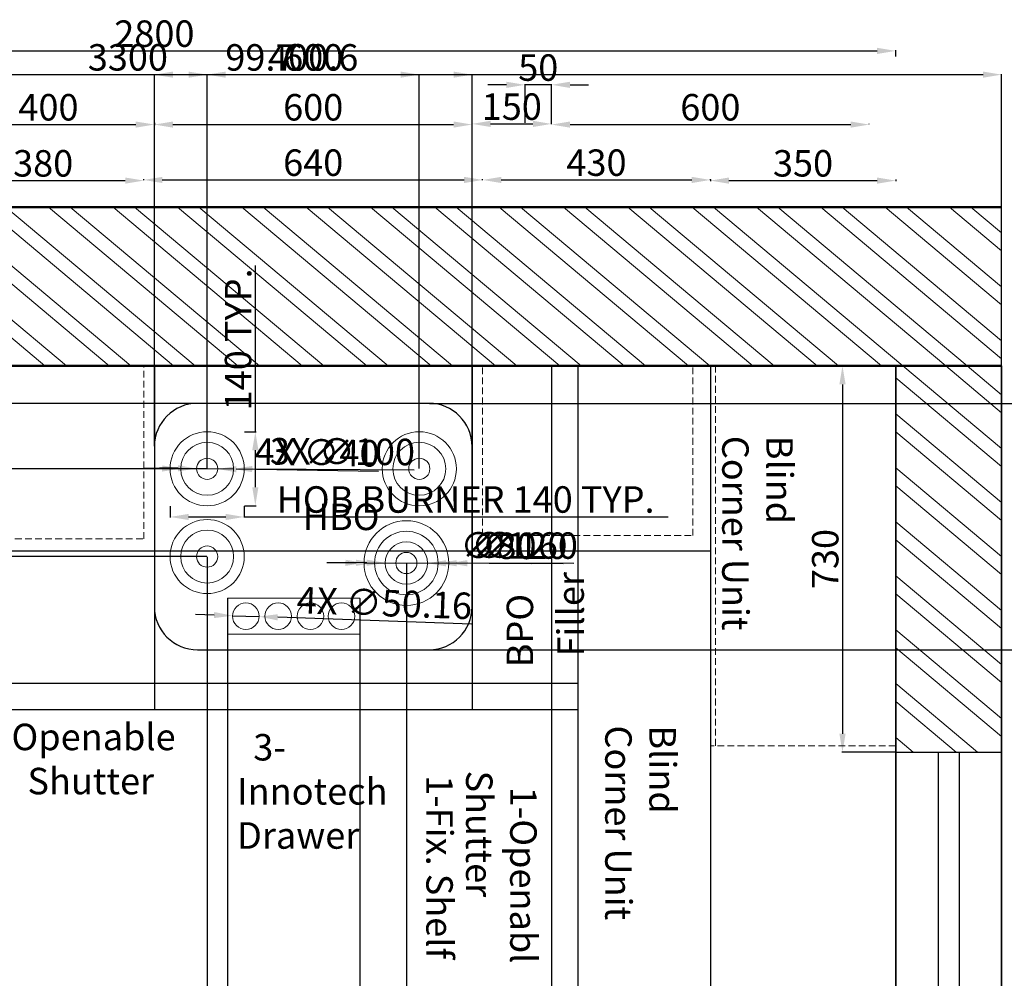
# Model space of a CAD drawing. Units: millimetres. Extents: x 407065 to 421840, y 1168257 to 1177792.
# Tile 9 of 17: x 409170 to 411029, y 1175981 to 1177792. Entities that reach past the tile are written whole.
import ezdxf

# ---------------------------------------------------------------- set-up
doc = ezdxf.new("R2010")
doc.units = ezdxf.units.MM
doc.linetypes.add('DASHED', pattern=[19.05, 12.7, -6.35])
for name, color, linetype, lineweight in [('A-ANNO-DIMS', 6, 'Continuous', 18), ('A-ANNO-TEXT', 30, 'Continuous', 18), ('A-EQPM', 8, 'Continuous', 18), ('A-FURN', 3, 'Continuous', 25), ('A-FURN-HIDN', 7, 'DASHED', 18), ('A-WALL', 7, 'Continuous', 50), ('A-WALL-PATT', 8, 'Continuous', 13)]:
    doc.layers.add(name, color=color, linetype=linetype, lineweight=lineweight)
doc.styles.get("Standard").update_dxf_attribs({"font": 'arial.ttf'})
doc.dimstyles.new('ISO-25', dxfattribs={"dimtxt": 50, "dimasz": 35, "dimexe": 1.25, "dimexo": 0.625, "dimtad": 1, "dimdec": 1, "dimtxsty": 'Standard', "dimcen": 35, "dimadec": 0, "dimazin": 0, "dimtfac": 1, "dimtdec": 1, "dimtmove": 0, "dimatfit": 3, "dimfxl": 1, "dimarcsym": 0})

# ---------------------------------------------------------------- blocks, each defined once
blk = doc.blocks.new('*D4')
at = {"layer": 'A-ANNO-DIMS', "color": 0, "lineweight": -2, "transparency": 16777216}
for p, q in [((409024.3, 1177488.3), (409024.3, 1177488.9)), ((409059.3, 1177487.7), (409369.3, 1177487.7)), ((409404.3, 1177488.3), (409404.3, 1177488.9))]:
    blk.add_line(p, q, dxfattribs=at)
at = {"layer": 'A-ANNO-DIMS', "color": 0, "transparency": 16777216}
for points in [[(409059.3, 1177493.5), (409059.3, 1177481.8), (409024.3, 1177487.7)], [(409369.3, 1177493.5), (409369.3, 1177481.8), (409404.3, 1177487.7)]]:
    blk.add_solid(points, dxfattribs=at)
at = {"layer": 'Defpoints', "color": 0, "transparency": 16777216}
for p in [(409024.3, 1177487.7), (409404.3, 1177487.7), (409404.3, 1177487.7)]:
    blk.add_point(p, dxfattribs=at)
at = {"layer": 'A-ANNO-DIMS', "color": 0, "transparency": 16777216, "insert": (409214.3, 1177513.8), "char_height": 50, "attachment_point": 5}
blk.add_mtext('380', dxfattribs=at)
blk = doc.blocks.new('*D5')
at = {"layer": 'A-ANNO-DIMS', "color": 0, "lineweight": -2, "transparency": 16777216}
for p, q in [((409404.3, 1177488.3), (409404.3, 1177490.2)), ((409439.3, 1177488.9), (410009.3, 1177488.9)), ((410044.3, 1177488.3), (410044.3, 1177490.2))]:
    blk.add_line(p, q, dxfattribs=at)
at = {"layer": 'A-ANNO-DIMS', "color": 0, "transparency": 16777216}
for points in [[(409439.3, 1177494.7), (409439.3, 1177483.1), (409404.3, 1177488.9)], [(410009.3, 1177494.7), (410009.3, 1177483.1), (410044.3, 1177488.9)]]:
    blk.add_solid(points, dxfattribs=at)
at = {"layer": 'Defpoints', "color": 0, "transparency": 16777216}
for p in [(409404.3, 1177487.7), (410044.3, 1177488.9), (410044.3, 1177487.7)]:
    blk.add_point(p, dxfattribs=at)
at = {"layer": 'A-ANNO-DIMS', "color": 0, "transparency": 16777216, "insert": (409724.3, 1177515.1), "char_height": 50, "attachment_point": 5}
blk.add_mtext('640', dxfattribs=at)
blk = doc.blocks.new('*D6')
at = {"layer": 'A-ANNO-DIMS', "color": 0, "lineweight": -2, "transparency": 16777216}
for p, q in [((410044.3, 1177488.3), (410044.3, 1177490.2)), ((410079.3, 1177488.9), (410439.3, 1177488.9)), ((410474.3, 1177488.3), (410474.3, 1177490.2))]:
    blk.add_line(p, q, dxfattribs=at)
at = {"layer": 'A-ANNO-DIMS', "color": 0, "transparency": 16777216}
for points in [[(410079.3, 1177494.7), (410079.3, 1177483.1), (410044.3, 1177488.9)], [(410439.3, 1177494.7), (410439.3, 1177483.1), (410474.3, 1177488.9)]]:
    blk.add_solid(points, dxfattribs=at)
at = {"layer": 'Defpoints', "color": 0, "transparency": 16777216}
for p in [(410044.3, 1177487.7), (410474.3, 1177488.9), (410474.3, 1177487.7)]:
    blk.add_point(p, dxfattribs=at)
at = {"layer": 'A-ANNO-DIMS', "color": 0, "transparency": 16777216, "insert": (410259.3, 1177515.1), "char_height": 50, "attachment_point": 5}
blk.add_mtext('430', dxfattribs=at)
blk = doc.blocks.new('*D7')
at = {"layer": 'A-ANNO-DIMS', "color": 0, "lineweight": -2, "transparency": 16777216}
for p, q in [((410474.3, 1177489.5), (410474.3, 1177486.4)), ((410509.3, 1177487.7), (410789.3, 1177487.7)), ((410824.3, 1177489.5), (410824.3, 1177486.4))]:
    blk.add_line(p, q, dxfattribs=at)
at = {"layer": 'A-ANNO-DIMS', "color": 0, "transparency": 16777216}
for points in [[(410509.3, 1177493.5), (410509.3, 1177481.8), (410474.3, 1177487.7)], [(410789.3, 1177493.5), (410789.3, 1177481.8), (410824.3, 1177487.7)]]:
    blk.add_solid(points, dxfattribs=at)
at = {"layer": 'Defpoints', "color": 0, "transparency": 16777216}
for p in [(410474.3, 1177490.2), (410824.3, 1177490.2), (410824.3, 1177487.7)]:
    blk.add_point(p, dxfattribs=at)
at = {"layer": 'A-ANNO-DIMS', "color": 0, "transparency": 16777216, "insert": (410649.3, 1177513.8), "char_height": 50, "attachment_point": 5}
blk.add_mtext('350', dxfattribs=at)
blk = doc.blocks.new('*D11')
at = {"layer": 'A-ANNO-DIMS', "color": 0, "lineweight": -2, "transparency": 16777216}
for p, q in [((409024.3, 1177596.6), (409024.3, 1177592.3)), ((409059.3, 1177593.5), (409389.3, 1177593.5)), ((409424.3, 1177596.6), (409424.3, 1177592.3))]:
    blk.add_line(p, q, dxfattribs=at)
at = {"layer": 'A-ANNO-DIMS', "color": 0, "transparency": 16777216}
for points in [[(409059.3, 1177599.3), (409059.3, 1177587.7), (409024.3, 1177593.5)], [(409389.3, 1177599.3), (409389.3, 1177587.7), (409424.3, 1177593.5)]]:
    blk.add_solid(points, dxfattribs=at)
at = {"layer": 'Defpoints', "color": 0, "transparency": 16777216}
for p in [(409024.3, 1177597.3), (409424.3, 1177597.3), (409424.3, 1177593.5)]:
    blk.add_point(p, dxfattribs=at)
at = {"layer": 'A-ANNO-DIMS', "color": 0, "transparency": 16777216, "insert": (409224.3, 1177619.7), "char_height": 50, "attachment_point": 5}
blk.add_mtext('400', dxfattribs=at)
blk = doc.blocks.new('*D12')
at = {"layer": 'A-ANNO-DIMS', "color": 0, "lineweight": -2, "transparency": 16777216}
for p, q in [((409424.3, 1177594.1), (409424.3, 1177594.8)), ((409459.3, 1177593.5), (409989.3, 1177593.5)), ((410024.3, 1177594.1), (410024.3, 1177594.8))]:
    blk.add_line(p, q, dxfattribs=at)
at = {"layer": 'A-ANNO-DIMS', "color": 0, "transparency": 16777216}
for points in [[(409459.3, 1177599.3), (409459.3, 1177587.7), (409424.3, 1177593.5)], [(409989.3, 1177599.3), (409989.3, 1177587.7), (410024.3, 1177593.5)]]:
    blk.add_solid(points, dxfattribs=at)
at = {"layer": 'Defpoints', "color": 0, "transparency": 16777216}
for p in [(409424.3, 1177593.5), (410024.3, 1177593.5), (410024.3, 1177593.5)]:
    blk.add_point(p, dxfattribs=at)
at = {"layer": 'A-ANNO-DIMS', "color": 0, "transparency": 16777216, "insert": (409724.3, 1177619.7), "char_height": 50, "attachment_point": 5}
blk.add_mtext('600', dxfattribs=at)
blk = doc.blocks.new('*D13')
at = {"layer": 'A-ANNO-DIMS', "color": 0, "lineweight": -2, "transparency": 16777216}
for p, q in [((410024.3, 1177594.1), (410024.3, 1177596)), ((410059.3, 1177594.8), (410139.3, 1177594.8)), ((410174.3, 1177594.1), (410174.3, 1177596))]:
    blk.add_line(p, q, dxfattribs=at)
at = {"layer": 'A-ANNO-DIMS', "color": 0, "transparency": 16777216}
for points in [[(410059.3, 1177600.6), (410059.3, 1177588.9), (410024.3, 1177594.8)], [(410139.3, 1177600.6), (410139.3, 1177588.9), (410174.3, 1177594.8)]]:
    blk.add_solid(points, dxfattribs=at)
at = {"layer": 'Defpoints', "color": 0, "transparency": 16777216}
for p in [(410024.3, 1177593.5), (410174.3, 1177594.8), (410174.3, 1177593.5)]:
    blk.add_point(p, dxfattribs=at)
at = {"layer": 'A-ANNO-DIMS', "color": 0, "transparency": 16777216, "insert": (410099.3, 1177620.9), "char_height": 50, "attachment_point": 5}
blk.add_mtext('150', dxfattribs=at)
blk = doc.blocks.new('*D14')
at = {"layer": 'A-ANNO-DIMS', "color": 0, "lineweight": -2, "transparency": 16777216}
for p, q in [((410089.3, 1177668.6), (410054.3, 1177668.6)), ((410124.3, 1177596.6), (410124.3, 1177669.8)), ((410174.3, 1177668.6), (410124.3, 1177668.6)), ((410174.3, 1177596.6), (410174.3, 1177669.8)), ((410209.3, 1177668.6), (410244.3, 1177668.6))]:
    blk.add_line(p, q, dxfattribs=at)
at = {"layer": 'A-ANNO-DIMS', "color": 0, "transparency": 16777216}
for points in [[(410089.3, 1177674.4), (410089.3, 1177662.7), (410124.3, 1177668.6)], [(410209.3, 1177674.4), (410209.3, 1177662.7), (410174.3, 1177668.6)]]:
    blk.add_solid(points, dxfattribs=at)
at = {"layer": 'Defpoints', "color": 0, "transparency": 16777216}
for p in [(410124.3, 1177668.6), (410124.3, 1177596), (410174.3, 1177596)]:
    blk.add_point(p, dxfattribs=at)
at = {"layer": 'A-ANNO-DIMS', "color": 0, "transparency": 16777216, "insert": (410149.3, 1177694.7), "char_height": 50, "attachment_point": 5}
blk.add_mtext('50', dxfattribs=at)
blk = doc.blocks.new('*D15')
at = {"layer": 'A-ANNO-DIMS', "color": 0, "lineweight": -2, "transparency": 16777216}
for p, q in [((410174.3, 1177594.1), (410174.3, 1177594.8)), ((410209.3, 1177593.5), (410739.3, 1177593.5)), ((410774.3, 1177594.1), (410774.3, 1177594.8))]:
    blk.add_line(p, q, dxfattribs=at)
at = {"layer": 'A-ANNO-DIMS', "color": 0, "transparency": 16777216}
for points in [[(410209.3, 1177599.3), (410209.3, 1177587.7), (410174.3, 1177593.5)], [(410739.3, 1177599.3), (410739.3, 1177587.7), (410774.3, 1177593.5)]]:
    blk.add_solid(points, dxfattribs=at)
at = {"layer": 'Defpoints', "color": 0, "transparency": 16777216}
for p in [(410174.3, 1177593.5), (410774.3, 1177593.5), (410774.3, 1177593.5)]:
    blk.add_point(p, dxfattribs=at)
at = {"layer": 'A-ANNO-DIMS', "color": 0, "transparency": 16777216, "insert": (410474.3, 1177619.7), "char_height": 50, "attachment_point": 5}
blk.add_mtext('600', dxfattribs=at)
blk = doc.blocks.new('*D16')
at = {"layer": 'A-ANNO-DIMS', "color": 0, "lineweight": -2, "transparency": 16777216}
for p, q in [((408024.3, 1177722.1), (408024.3, 1177733.9)), ((410824.3, 1177722.1), (410824.3, 1177733.9)), ((408059.3, 1177732.7), (410789.3, 1177732.7))]:
    blk.add_line(p, q, dxfattribs=at)
at = {"layer": 'A-ANNO-DIMS', "color": 0, "transparency": 16777216}
for points in [[(408059.3, 1177738.5), (408059.3, 1177726.8), (408024.3, 1177732.7)], [(410789.3, 1177738.5), (410789.3, 1177726.8), (410824.3, 1177732.7)]]:
    blk.add_solid(points, dxfattribs=at)
at = {"layer": 'Defpoints', "color": 0, "transparency": 16777216}
for p in [(408024.3, 1177721.4), (410824.3, 1177732.7), (410824.3, 1177721.4)]:
    blk.add_point(p, dxfattribs=at)
at = {"layer": 'A-ANNO-DIMS', "color": 0, "transparency": 16777216, "insert": (409424.3, 1177758.8), "char_height": 50, "attachment_point": 5}
blk.add_mtext('2800', dxfattribs=at)
blk = doc.blocks.new('*D17')
at = {"layer": 'A-ANNO-DIMS', "color": 0, "lineweight": -2, "transparency": 16777216}
for p, q in [((410828.1, 1177137.8), (410722.6, 1177137.8)), ((410723.8, 1177102.8), (410723.8, 1176442.8)), ((410823.7, 1176407.8), (410722.6, 1176407.8))]:
    blk.add_line(p, q, dxfattribs=at)
at = {"layer": 'A-ANNO-DIMS', "color": 0, "transparency": 16777216}
for points in [[(410718, 1177102.8), (410729.7, 1177102.8), (410723.8, 1177137.8)], [(410718, 1176442.8), (410729.7, 1176442.8), (410723.8, 1176407.8)]]:
    blk.add_solid(points, dxfattribs=at)
at = {"layer": 'Defpoints', "color": 0, "transparency": 16777216}
for p in [(410828.7, 1177137.8), (410723.8, 1176407.8), (410824.3, 1176407.8)]:
    blk.add_point(p, dxfattribs=at)
at = {"layer": 'A-ANNO-DIMS', "color": 0, "transparency": 16777216, "insert": (410697.7, 1176772.8), "char_height": 50, "attachment_point": 5, "rotation": 90}
blk.add_mtext('730', dxfattribs=at)
blk = doc.blocks.new('HOB-BURNER')
for radius in [70, 50, 20]:
    blk.add_circle((409524, 1176943.3), radius)
blk = doc.blocks.new('*D161')
at = {"layer": 'A-ANNO-DIMS', "color": 0, "lineweight": -2, "transparency": 16777216}
for p, q in [((409454, 1176872.7), (409454, 1176851.1)), ((409594, 1176872.7), (409594, 1176851.1)), ((409489, 1176852.3), (409559, 1176852.3)), ((409594, 1176852.3), (410394.9, 1176852.3))]:
    blk.add_line(p, q, dxfattribs=at)
at = {"layer": 'A-ANNO-DIMS', "color": 0, "transparency": 16777216}
for points in [[(409489, 1176858.1), (409489, 1176846.5), (409454, 1176852.3)], [(409559, 1176858.1), (409559, 1176846.5), (409594, 1176852.3)]]:
    blk.add_solid(points, dxfattribs=at)
at = {"layer": 'Defpoints', "color": 0, "transparency": 16777216}
for p in [(409454, 1176873.3), (409594, 1176873.3), (409594, 1176852.3)]:
    blk.add_point(p, dxfattribs=at)
at = {"layer": 'A-ANNO-DIMS', "color": 0, "transparency": 16777216, "insert": (410012, 1176878.8), "char_height": 50, "attachment_point": 5}
blk.add_mtext('HOB BURNER 140 TYP.', dxfattribs=at)
blk = doc.blocks.new('*D162')
at = {"layer": 'A-ANNO-DIMS', "color": 0, "lineweight": -2, "transparency": 16777216}
for p, q in [((409615, 1177013.3), (409615, 1177327.1)), ((409594.6, 1177013.3), (409616.3, 1177013.3)), ((409615, 1176908.3), (409615, 1176978.3)), ((409594.6, 1176873.3), (409616.3, 1176873.3))]:
    blk.add_line(p, q, dxfattribs=at)
at = {"layer": 'A-ANNO-DIMS', "color": 0, "transparency": 16777216}
for points in [[(409609.2, 1176978.3), (409620.8, 1176978.3), (409615, 1177013.3)], [(409609.2, 1176908.3), (409620.8, 1176908.3), (409615, 1176873.3)]]:
    blk.add_solid(points, dxfattribs=at)
at = {"layer": 'Defpoints', "color": 0, "transparency": 16777216}
for p in [(409594, 1177013.3), (409615, 1177013.3), (409594, 1176873.3)]:
    blk.add_point(p, dxfattribs=at)
at = {"layer": 'A-ANNO-DIMS', "color": 0, "transparency": 16777216, "insert": (409588.9, 1177187.7), "char_height": 50, "attachment_point": 5, "rotation": 90}
blk.add_mtext('140 TYP.', dxfattribs=at)
blk = doc.blocks.new('*D165')
at = {"layer": 'A-ANNO-DIMS', "color": 0, "lineweight": -2, "transparency": 16777216}
for p, q in [((407724.3, 1177438.4), (407724.3, 1177689)), ((407759.3, 1177687.8), (410989.3, 1177687.8)), ((411024.3, 1177438.4), (411024.3, 1177689))]:
    blk.add_line(p, q, dxfattribs=at)
at = {"layer": 'A-ANNO-DIMS', "color": 0, "transparency": 16777216}
for points in [[(407759.3, 1177693.6), (407759.3, 1177682), (407724.3, 1177687.8)], [(410989.3, 1177693.6), (410989.3, 1177682), (411024.3, 1177687.8)]]:
    blk.add_solid(points, dxfattribs=at)
at = {"layer": 'Defpoints', "color": 0, "transparency": 16777216}
for p in [(411024.3, 1177687.8), (407724.3, 1177437.8), (411024.3, 1177437.8)]:
    blk.add_point(p, dxfattribs=at)
at = {"layer": 'A-ANNO-DIMS', "color": 0, "transparency": 16777216, "insert": (409374.3, 1177714), "char_height": 50, "attachment_point": 5}
blk.add_mtext('3300', dxfattribs=at)
blk = doc.blocks.new('*D178')
at = {"layer": 'A-ANNO-DIMS', "color": 0, "lineweight": -2, "transparency": 16777216}
for p, q in [((409424.3, 1176986.1), (409424.3, 1177689)), ((409459.3, 1177687.8), (409989.3, 1177687.8)), ((410024.3, 1176986.1), (410024.3, 1177689))]:
    blk.add_line(p, q, dxfattribs=at)
at = {"layer": 'A-ANNO-DIMS', "color": 0, "transparency": 16777216}
for points in [[(409459.3, 1177693.6), (409459.3, 1177682), (409424.3, 1177687.8)], [(409989.3, 1177693.6), (409989.3, 1177682), (410024.3, 1177687.8)]]:
    blk.add_solid(points, dxfattribs=at)
at = {"layer": 'Defpoints', "color": 0, "transparency": 16777216}
for p in [(410024.3, 1177687.8), (409424.3, 1176985.5), (410024.3, 1176985.5)]:
    blk.add_point(p, dxfattribs=at)
at = {"layer": 'A-ANNO-DIMS', "color": 0, "transparency": 16777216, "insert": (409724.3, 1177713.9), "char_height": 50, "attachment_point": 5}
blk.add_mtext('600', dxfattribs=at)
blk = doc.blocks.new('*D179')
at = {"layer": 'A-ANNO-DIMS', "color": 0, "lineweight": -2, "transparency": 16777216}
for p, q in [((409943.6, 1177066.8), (411961.4, 1177066.8)), ((411960.2, 1177031.8), (411960.2, 1176636.4)), ((409943.6, 1176601.4), (411961.4, 1176601.4))]:
    blk.add_line(p, q, dxfattribs=at)
at = {"layer": 'A-ANNO-DIMS', "color": 0, "transparency": 16777216}
for points in [[(411954.3, 1177031.8), (411966, 1177031.8), (411960.2, 1177066.8)], [(411954.3, 1176636.4), (411966, 1176636.4), (411960.2, 1176601.4)]]:
    blk.add_solid(points, dxfattribs=at)
at = {"layer": 'Defpoints', "color": 0, "transparency": 16777216}
for p in [(409943, 1177066.8), (409943, 1176601.4), (411960.2, 1176601.4)]:
    blk.add_point(p, dxfattribs=at)
at = {"layer": 'A-ANNO-DIMS', "color": 0, "transparency": 16777216, "insert": (411934, 1176834.1), "char_height": 50, "attachment_point": 5, "rotation": 90}
blk.add_mtext('465.4', dxfattribs=at)
blk = doc.blocks.new('*D180')
at = {"layer": 'A-ANNO-DIMS', "color": 0, "lineweight": -2, "transparency": 16777216}
for p, q in [((409424.3, 1176986.1), (409424.3, 1177689)), ((409459.3, 1177687.8), (409489, 1177687.8)), ((409524, 1176943.9), (409524, 1177689)), ((409524, 1177687.8), (409690.1, 1177687.8))]:
    blk.add_line(p, q, dxfattribs=at)
at = {"layer": 'A-ANNO-DIMS', "color": 0, "transparency": 16777216}
for points in [[(409459.3, 1177693.6), (409459.3, 1177682), (409424.3, 1177687.8)], [(409489, 1177693.6), (409489, 1177682), (409524, 1177687.8)]]:
    blk.add_solid(points, dxfattribs=at)
at = {"layer": 'Defpoints', "color": 0, "transparency": 16777216}
for p in [(409524, 1177687.8), (409424.3, 1176985.5), (409524, 1176943.3)]:
    blk.add_point(p, dxfattribs=at)
at = {"layer": 'A-ANNO-DIMS', "color": 0, "transparency": 16777216, "insert": (409624.6, 1177713.9), "char_height": 50, "attachment_point": 5}
blk.add_mtext('99.7', dxfattribs=at)
blk = doc.blocks.new('*D181')
at = {"layer": 'A-ANNO-DIMS', "color": 0, "lineweight": -2, "transparency": 16777216}
for p, q in [((409524, 1176943.9), (409524, 1177689)), ((409559, 1177687.8), (409889.6, 1177687.8)), ((409924.6, 1176943.9), (409924.6, 1177689))]:
    blk.add_line(p, q, dxfattribs=at)
at = {"layer": 'A-ANNO-DIMS', "color": 0, "transparency": 16777216}
for points in [[(409559, 1177693.6), (409559, 1177682), (409524, 1177687.8)], [(409889.6, 1177693.6), (409889.6, 1177682), (409924.6, 1177687.8)]]:
    blk.add_solid(points, dxfattribs=at)
at = {"layer": 'Defpoints', "color": 0, "transparency": 16777216}
for p in [(409924.6, 1177687.8), (409524, 1176943.3), (409924.6, 1176943.3)]:
    blk.add_point(p, dxfattribs=at)
at = {"layer": 'A-ANNO-DIMS', "color": 0, "transparency": 16777216, "insert": (409724.3, 1177713.9), "char_height": 50, "attachment_point": 5}
blk.add_mtext('400.6', dxfattribs=at)
blk = doc.blocks.new('*D182')
at = {"layer": 'A-ANNO-DIMS', "color": 0, "lineweight": -2, "transparency": 16777216}
for p, q in [((409505, 1177066.8), (407473.1, 1177066.8)), ((407474.3, 1177031.8), (407474.3, 1176978.3)), ((409523.4, 1176943.3), (407473.1, 1176943.3)), ((407474.3, 1176943.3), (407474.3, 1176742.7))]:
    blk.add_line(p, q, dxfattribs=at)
at = {"layer": 'A-ANNO-DIMS', "color": 0, "transparency": 16777216}
for points in [[(407468.5, 1177031.8), (407480.1, 1177031.8), (407474.3, 1177066.8)], [(407468.5, 1176978.3), (407480.1, 1176978.3), (407474.3, 1176943.3)]]:
    blk.add_solid(points, dxfattribs=at)
at = {"layer": 'Defpoints', "color": 0, "transparency": 16777216}
for p in [(409505.7, 1177066.8), (407474.3, 1176943.3), (409524, 1176943.3)]:
    blk.add_point(p, dxfattribs=at)
at = {"layer": 'A-ANNO-DIMS', "color": 0, "transparency": 16777216, "insert": (407448.1, 1176825.5), "char_height": 50, "attachment_point": 5, "rotation": 90}
blk.add_mtext('123.5', dxfattribs=at)
blk = doc.blocks.new('*D183')
at = {"layer": 'A-ANNO-DIMS', "color": 0, "lineweight": -2, "transparency": 16777216}
for p, q in [((409523.4, 1176943.3), (407473.1, 1176943.3)), ((407474.3, 1176908.3), (407474.3, 1176812.5)), ((409523.4, 1176777.5), (407473.1, 1176777.5)), ((407474.3, 1176777.5), (407474.3, 1176538.4))]:
    blk.add_line(p, q, dxfattribs=at)
at = {"layer": 'A-ANNO-DIMS', "color": 0, "transparency": 16777216}
for points in [[(407468.5, 1176908.3), (407480.1, 1176908.3), (407474.3, 1176943.3)], [(407468.5, 1176812.5), (407480.1, 1176812.5), (407474.3, 1176777.5)]]:
    blk.add_solid(points, dxfattribs=at)
at = {"layer": 'Defpoints', "color": 0, "transparency": 16777216}
for p in [(409524, 1176943.3), (407474.3, 1176777.5), (409524, 1176777.5)]:
    blk.add_point(p, dxfattribs=at)
at = {"layer": 'A-ANNO-DIMS', "color": 0, "transparency": 16777216, "insert": (407448.2, 1176640.4), "char_height": 50, "attachment_point": 5, "rotation": 90}
blk.add_mtext('165.86', dxfattribs=at)
blk = doc.blocks.new('*D184')
at = {"layer": 'A-ANNO-DIMS', "color": 0, "lineweight": -2, "transparency": 16777216}
for p, q in [((409524, 1176776.8), (409524, 1172896.5)), ((409900.3, 1176764.7), (409900.3, 1172896.5)), ((409559, 1172897.8), (409865.3, 1172897.8))]:
    blk.add_line(p, q, dxfattribs=at)
at = {"layer": 'A-ANNO-DIMS', "color": 0, "transparency": 16777216}
for points in [[(409559, 1172903.6), (409559, 1172892), (409524, 1172897.8)], [(409865.3, 1172903.6), (409865.3, 1172892), (409900.3, 1172897.8)]]:
    blk.add_solid(points, dxfattribs=at)
at = {"layer": 'Defpoints', "color": 0, "transparency": 16777216}
for p in [(409524, 1176777.5), (409900.3, 1176765.3), (409900.3, 1172897.8)]:
    blk.add_point(p, dxfattribs=at)
at = {"layer": 'A-ANNO-DIMS', "color": 0, "transparency": 16777216, "insert": (409712.1, 1172924), "char_height": 50, "attachment_point": 5}
blk.add_mtext('376.24', dxfattribs=at)
blk = doc.blocks.new('*D185')
at = {"layer": 'A-ANNO-DIMS', "color": 0, "lineweight": -2, "transparency": 16777216}
for p, q in [((409562.3, 1176698.3), (409562.3, 1172896.5)), ((409812.5, 1176698.3), (409812.5, 1172896.5)), ((409597.3, 1172897.8), (409777.5, 1172897.8))]:
    blk.add_line(p, q, dxfattribs=at)
at = {"layer": 'A-ANNO-DIMS', "color": 0, "transparency": 16777216}
for points in [[(409597.3, 1172903.6), (409597.3, 1172892), (409562.3, 1172897.8)], [(409777.5, 1172903.6), (409777.5, 1172892), (409812.5, 1172897.8)]]:
    blk.add_solid(points, dxfattribs=at)
at = {"layer": 'Defpoints', "color": 0, "transparency": 16777216}
for p in [(409562.3, 1176698.9), (409812.5, 1176698.9), (409812.5, 1172897.8)]:
    blk.add_point(p, dxfattribs=at)
at = {"layer": 'A-ANNO-DIMS', "color": 0, "transparency": 16777216, "insert": (409687.4, 1172923.9), "char_height": 50, "attachment_point": 5}
blk.add_mtext('250.25', dxfattribs=at)
blk = doc.blocks.new('*D224')
at = {"layer": 'A-ANNO-DIMS', "color": 0, "lineweight": -2, "transparency": 16777216}
for p, q in [((409785.3, 1176765.7), (409750.3, 1176765.8)), ((409820.3, 1176765.6), (409980.3, 1176765)), ((410216.2, 1176764.2), (410015.3, 1176764.9))]:
    blk.add_line(p, q, dxfattribs=at)
at = {"layer": 'A-ANNO-DIMS', "color": 0, "transparency": 16777216}
for points in [[(409785.3, 1176771.5), (409785.2, 1176759.8), (409820.3, 1176765.6)], [(410015.3, 1176770.7), (410015.2, 1176759), (409980.3, 1176765)]]:
    blk.add_solid(points, dxfattribs=at)
at = {"layer": 'Defpoints', "color": 0, "transparency": 16777216}
for p in [(409820.3, 1176765.6), (409980.3, 1176765)]:
    blk.add_point(p, dxfattribs=at)
at = {"layer": 'A-ANNO-DIMS', "color": 0, "transparency": 16777216, "insert": (410133.3, 1176792), "char_height": 50, "attachment_point": 5, "rotation": 359.802}
blk.add_mtext('∅160', dxfattribs=at)
blk = doc.blocks.new('*D225')
at = {"layer": 'A-ANNO-DIMS', "color": 0, "lineweight": -2, "transparency": 16777216}
for p, q in [((409805.3, 1176765.7), (409770.3, 1176765.9)), ((409840.3, 1176765.6), (409960.3, 1176765)), ((410196.2, 1176763.9), (409995.3, 1176764.8))]:
    blk.add_line(p, q, dxfattribs=at)
at = {"layer": 'A-ANNO-DIMS', "color": 0, "transparency": 16777216}
for points in [[(409805.3, 1176771.5), (409805.2, 1176759.9), (409840.3, 1176765.6)], [(409995.3, 1176770.7), (409995.2, 1176759), (409960.3, 1176765)]]:
    blk.add_solid(points, dxfattribs=at)
at = {"layer": 'Defpoints', "color": 0, "transparency": 16777216}
for p in [(409840.3, 1176765.6), (409960.3, 1176765)]:
    blk.add_point(p, dxfattribs=at)
at = {"layer": 'A-ANNO-DIMS', "color": 0, "transparency": 16777216, "insert": (410113.4, 1176791.8), "char_height": 50, "attachment_point": 5, "rotation": 359.7357}
blk.add_mtext('∅120', dxfattribs=at)
blk = doc.blocks.new('*D226')
at = {"layer": 'A-ANNO-DIMS', "color": 0, "lineweight": -2, "transparency": 16777216}
for p, q in [((409825.3, 1176765.8), (409790.3, 1176766)), ((409860.3, 1176765.6), (409940.3, 1176765)), ((410137.4, 1176763.6), (409975.3, 1176764.8))]:
    blk.add_line(p, q, dxfattribs=at)
at = {"layer": 'A-ANNO-DIMS', "color": 0, "transparency": 16777216}
for points in [[(409825.3, 1176771.6), (409825.2, 1176760), (409860.3, 1176765.6)], [(409975.3, 1176770.6), (409975.2, 1176758.9), (409940.3, 1176765)]]:
    blk.add_solid(points, dxfattribs=at)
at = {"layer": 'Defpoints', "color": 0, "transparency": 16777216}
for p in [(409860.3, 1176765.6), (409940.3, 1176765)]:
    blk.add_point(p, dxfattribs=at)
at = {"layer": 'A-ANNO-DIMS', "color": 0, "transparency": 16777216, "insert": (410074, 1176791.6), "char_height": 50, "attachment_point": 5, "rotation": 359.6026}
blk.add_mtext('∅80', dxfattribs=at)
blk = doc.blocks.new('*D227')
at = {"layer": 'A-ANNO-DIMS', "color": 0, "lineweight": -2, "transparency": 16777216}
for p, q in [((409439, 1176943.9), (409404, 1176944.1)), ((409474, 1176943.6), (409574, 1176943)), ((409914.7, 1176940.8), (409609, 1176942.8))]:
    blk.add_line(p, q, dxfattribs=at)
at = {"layer": 'A-ANNO-DIMS', "color": 0, "transparency": 16777216}
for points in [[(409439.1, 1176949.7), (409439, 1176938), (409474, 1176943.6)], [(409609.1, 1176948.6), (409609, 1176936.9), (409574, 1176943)]]:
    blk.add_solid(points, dxfattribs=at)
at = {"layer": 'Defpoints', "color": 0, "transparency": 16777216}
for p in [(409474, 1176943.6), (409574, 1176943)]:
    blk.add_point(p, dxfattribs=at)
at = {"layer": 'A-ANNO-DIMS', "color": 0, "transparency": 16777216, "insert": (409779.5, 1176969.3), "char_height": 50, "attachment_point": 5, "rotation": 359.6376}
blk.add_mtext('3X ∅100', dxfattribs=at)
blk = doc.blocks.new('*D228')
at = {"layer": 'A-ANNO-DIMS', "color": 0, "lineweight": -2, "transparency": 16777216}
for p, q in [((409469, 1176944.2), (409434, 1176944.7)), ((409504, 1176943.6), (409544, 1176943)), ((409847.9, 1176938.2), (409579, 1176942.4))]:
    blk.add_line(p, q, dxfattribs=at)
at = {"layer": 'A-ANNO-DIMS', "color": 0, "transparency": 16777216}
for points in [[(409469.1, 1176950), (409468.9, 1176938.4), (409504, 1176943.6)], [(409579.1, 1176948.3), (409578.9, 1176936.6), (409544, 1176943)]]:
    blk.add_solid(points, dxfattribs=at)
at = {"layer": 'Defpoints', "color": 0, "transparency": 16777216}
for p in [(409504, 1176943.6), (409544, 1176943)]:
    blk.add_point(p, dxfattribs=at)
at = {"layer": 'A-ANNO-DIMS', "color": 0, "transparency": 16777216, "insert": (409731.4, 1176967.6), "char_height": 50, "attachment_point": 5, "rotation": 359.0937}
blk.add_mtext('4X ∅40', dxfattribs=at)
blk = doc.blocks.new('*D231')
at = {"layer": 'A-ANNO-DIMS', "color": 0, "lineweight": -2, "transparency": 16777216}
for p, q in [((409537.1, 1176667), (409502.1, 1176668.2)), ((409572.1, 1176665.8), (409622.2, 1176664)), ((410023.1, 1176649.9), (409657.2, 1176662.8))]:
    blk.add_line(p, q, dxfattribs=at)
at = {"layer": 'A-ANNO-DIMS', "color": 0, "transparency": 16777216}
for points in [[(409537.3, 1176672.8), (409536.9, 1176661.2), (409572.1, 1176665.8)], [(409657.4, 1176668.6), (409657, 1176656.9), (409622.2, 1176664)]]:
    blk.add_solid(points, dxfattribs=at)
at = {"layer": 'Defpoints', "color": 0, "transparency": 16777216}
for p in [(409572.1, 1176665.8), (409622.2, 1176664)]:
    blk.add_point(p, dxfattribs=at)
at = {"layer": 'A-ANNO-DIMS', "color": 0, "transparency": 16777216, "insert": (409858.6, 1176683.3), "char_height": 50, "attachment_point": 5, "rotation": 357.9867}
blk.add_mtext('4X ∅50.16', dxfattribs=at)

msp = doc.modelspace()

# ---------------------------------------------------------------- hatches: boundary and pattern name
at = {"layer": 'A-WALL-PATT'}
h = msp.add_hatch(dxfattribs=at)
h.set_pattern_fill('ANSI32', color=256, scale=8.2, angle=95)
h.paths.add_polyline_path([(411024.3133, 1177437.7952), (407724.3133, 1177437.7952), (407724.3133, 1177137.7952), (408024.3133, 1177137.7952), (410824.3133, 1177137.7952), (411024.3133, 1177137.7952)])
h = msp.add_hatch(dxfattribs=at)
h.set_pattern_fill('ANSI32', color=256, scale=8.2, angle=95)
h.paths.add_polyline_path([(411024.3133, 1177137.7952), (410824.3133, 1177137.7952), (410824.3133, 1176407.7952), (411024.3133, 1176407.7952)])

# ---------------------------------------------------------------- linework, layer by layer
at = {"layer": 'A-EQPM'}
msp.add_lwpolyline([(409562.2649, 1176698.8834), (409812.5157, 1176698.8834), (409812.5157, 1176630.8621), (409562.2649, 1176630.8621)], close=True, dxfattribs=at)
for centre, radius in [((409900.2591, 1176765.2756), 80), ((409900.2591, 1176765.2756), 60), ((409900.2591, 1176765.2756), 40), ((409900.2591, 1176765.2756), 20), ((409597.1727, 1176664.8727), 25.0815), ((409658.1191, 1176664.8727), 25.0815), ((409719.0314, 1176664.8727), 25.0815), ((409777.7101, 1176664.8727), 25.0815)]:
    msp.add_circle(centre, radius, dxfattribs=at)
at = {"layer": 'A-FURN'}
for p, q in [((411024.3133, 1174717.7952), (411024.3133, 1177437.7952)), ((409424.3133, 1177137.7952), (409424.3133, 1176487.7952)), ((410024.3133, 1177137.7952), (410024.3133, 1176487.7952)), ((410174.3133, 1177137.7952), (410174.3133, 1174737.7952)), ((410224.3133, 1177137.7952), (410224.3133, 1174737.7952)), ((410474.3133, 1177137.7952), (410474.3133, 1174737.7952)), ((410824.3133, 1177137.7952), (410824.3133, 1174717.7952)), ((410824.3133, 1174717.7952), (410824.3133, 1177137.7952)), ((411024.3133, 1177137.7952), (411024.3133, 1174717.7952)), ((410474.3133, 1176787.7952), (408374.3133, 1176787.7952)), ((410224.3133, 1176537.7952), (408524.3133, 1176537.7952)), ((410224.3133, 1176487.7952), (408524.3133, 1176487.7952)), ((410904.3133, 1176407.7952), (410904.3133, 1175477.7952)), ((410944.3133, 1176407.7952), (410944.3133, 1175477.7952))]:
    msp.add_line(p, q, dxfattribs=at)
for points in [[(409942.9713, 1177066.8168), (409505.6554, 1177066.8168, 0.414213562), (409424.3133, 1176985.4747)], [(410024.3133, 1176682.7483), (410024.3133, 1176985.4747, 0.414213562), (409942.9713, 1177066.8168)], [(409424.3133, 1176985.4747), (409424.3133, 1176682.7483, 0.414213562), (409505.6554, 1176601.4062)], [(409505.6554, 1176601.4062), (409942.9713, 1176601.4062, 0.414213562), (410024.3133, 1176682.7483)]]:
    msp.add_lwpolyline(points, format="xyb", dxfattribs=at)
msp.add_lwpolyline([(410824.3133, 1176407.7952), (411024.3133, 1176407.7952), (411024.3133, 1175477.7952), (410824.3133, 1175477.7952)], close=True, dxfattribs=at)
at = {"layer": 'A-FURN-HIDN'}
for p, q in [((409404.3149, 1176811.0044), (409404.3149, 1177137.7952)), ((410044.3149, 1176817.3455), (410044.3149, 1177137.7952)), ((410441.4631, 1176817.3455), (410441.4631, 1177137.7952)), ((410484.3133, 1177137.7952), (410484.3133, 1176419.9871)), ((408646.6902, 1176811.0192), (409404.3149, 1176811.0044)), ((410044.3149, 1176817.3455), (410441.4631, 1176817.3455)), ((410824.3133, 1176419.9871), (410474.3133, 1176419.9871))]:
    msp.add_line(p, q, dxfattribs=at)
at = {"layer": 'A-WALL'}
for p, q in [((411024.3133, 1177437.7952), (407724.3133, 1177437.7952)), ((410824.3133, 1177137.7952), (408024.3133, 1177137.7952)), ((410824.3133, 1177137.7952), (411024.3133, 1177137.7952))]:
    msp.add_line(p, q, dxfattribs=at)

# ---------------------------------------------------------------- block references
at = {"layer": 'A-EQPM'}
for p in [(0, 0), (400.5954, 0), (0, -165.8625)]:
    msp.add_blockref('HOB-BURNER', p, dxfattribs=at)

# ---------------------------------------------------------------- texts
at = {"layer": 'A-ANNO-TEXT', "char_height": 50, "attachment_point": 1}
for s, width, insert, rotation in [('Blind Corner Unit', 382.409863, (410630.0286, 1177005.5683), 270), ('     Filler', 382.409863, (410185.397, 1176512.3886), 90), ('  BPO', 382.409863, (410089.5949, 1176537.7952), 90), ('Blind Corner Unit', 382.409863, (410409.1375, 1176458.4622), 270), (' 1-Fix. Shelf', 382.409863, (409987.8815, 1176379.7197), 270), ('  1-Openabl Shutter', 534.084465, (410146.2728, 1176373.2573), 270)]:
    msp.add_mtext_dynamic_manual_height_columns(s, width=width, gutter_width=12.5, heights=[0], dxfattribs=dict(at, insert=insert, rotation=rotation))
for s, insert in [('HBO', (409704.4285, 1176877.4788)), ('  1-Openable\\P      Shutter', (409092.9692, 1176461.7378)), ('  3- Innotech Drawer', (409580.4835, 1176442.255))]:
    msp.add_mtext_dynamic_manual_height_columns(s, width=382.409863, gutter_width=12.5, heights=[0], dxfattribs=dict(at, insert=insert))

# ---------------------------------------------------------------- dimensions: what is measured, and where the dimension line sits
at = {"layer": 'A-ANNO-DIMS'}
for base, p1, p2, override, picture, middle in [((410824.3133, 1177732.6671), (408024.3133, 1177721.4288), (410824.3133, 1177721.4288), {"dimclrd": 0, "dimclre": 0, "dimclrt": 0}, '*D16', (409424.3133, 1177758.8207)), ((411024.3133, 1177687.7952), (407724.3133, 1177437.7952), (411024.3133, 1177437.7952), {"dimdec": 0, "dimlfac": 1, "dimrnd": 0, "dimzin": 0, "dimdsep": 46, "dimlunit": 2}, '*D165', (409374.3133, 1177713.9659)), ((410024.3133, 1177687.7952), (409424.3133, 1176985.4747), (410024.3133, 1176985.4747), {"dimdec": 0, "dimlfac": 1, "dimrnd": 0, "dimzin": 0, "dimdsep": 46, "dimlunit": 2}, '*D178', (409724.3133, 1177713.9489)), ((409524.0157, 1177687.7952), (409424.3133, 1176985.4747), (409524.0157, 1176943.3161), {"dimdec": 1, "dimlfac": 1, "dimrnd": 0, "dimzin": 0, "dimdsep": 46, "dimlunit": 2}, '*D180', (409624.5793, 1177713.9489)), ((409924.611, 1177687.7952), (409524.0157, 1176943.3161), (409924.611, 1176943.3161), {"dimdec": 1, "dimlfac": 1, "dimrnd": 0, "dimzin": 0, "dimdsep": 46, "dimlunit": 2}, '*D181', (409724.3133, 1177713.9489)), ((409424.3133, 1177593.5123), (409024.3133, 1177597.2623), (409424.3133, 1177597.2623), {"dimclrd": 0, "dimclre": 0, "dimclrt": 0}, '*D11', (409224.3133, 1177619.666)), ((410024.3133, 1177593.5123), (409424.3133, 1177593.5123), (410024.3133, 1177593.5123), {"dimclrd": 0, "dimclre": 0, "dimclrt": 0}, '*D12', (409724.3133, 1177619.666)), ((410174.3133, 1177594.7623), (410024.3133, 1177593.5123), (410174.3133, 1177593.5123), {"dimclrd": 0, "dimclre": 0, "dimclrt": 0}, '*D13', (410099.3133, 1177620.916)), ((410774.3133, 1177593.5123), (410174.3133, 1177593.5123), (410774.3133, 1177593.5123), {"dimclrd": 0, "dimclre": 0, "dimclrt": 0}, '*D15', (410474.3133, 1177619.666)), ((410044.3149, 1177488.9032), (409404.3149, 1177487.6532), (410044.3149, 1177487.6532), {"dimclrd": 0, "dimclre": 0, "dimclrt": 0}, '*D5', (409724.3149, 1177515.0568)), ((410474.3133, 1177488.9032), (410044.3149, 1177487.6532), (410474.3133, 1177487.6532), {"dimclrd": 0, "dimclre": 0, "dimclrt": 0}, '*D6', (410259.3141, 1177515.0739)), ((409404.3149, 1177487.6532), (409024.3133, 1177487.6532), (409404.3149, 1177487.6532), {"dimclrd": 0, "dimclre": 0, "dimclrt": 0}, '*D4', (409214.3141, 1177513.8239)), ((410824.3133, 1177487.6532), (410474.3133, 1177490.1532), (410824.3133, 1177490.1532), {"dimclrd": 0, "dimclre": 0, "dimclrt": 0}, '*D7', (410649.3133, 1177513.8239)), ((409900.2591, 1172897.7952), (409524.0157, 1176777.4536), (409900.2591, 1176765.2756), {"dimdec": 2, "dimlfac": 1, "dimrnd": 0, "dimzin": 0, "dimdsep": 46, "dimlunit": 2}, '*D184', (409712.1374, 1172923.9659)), ((409812.5157, 1172897.7952), (409562.2649, 1176698.8834), (409812.5157, 1176698.8834), {"dimdec": 2, "dimlfac": 1, "dimrnd": 0, "dimzin": 0, "dimdsep": 46, "dimlunit": 2}, '*D185', (409687.3903, 1172923.9489))]:
    dim = msp.add_linear_dim(base=base, p1=p1, p2=p2, dimstyle='ISO-25', override=override, dxfattribs=at)
    dim.commit()
    dim.dimension.update_dxf_attribs({"geometry": picture, "text_midpoint": middle})
dim = msp.add_linear_dim(base=(410124.3133, 1177668.5564), p1=(410174.3133, 1177596.0123), p2=(410124.3133, 1177596.0123), dimstyle='ISO-25', override={"dimclrd": 0, "dimclre": 0, "dimclrt": 0}, dxfattribs=at)
dim.commit()
dim.dimension.update_dxf_attribs({"geometry": '*D14', "text_midpoint": (410149.3133, 1177668.5564), "dimtype": 160})
dim = msp.add_linear_dim(base=(409615.0157, 1177013.3161), p1=(409594.0157, 1176873.3161), p2=(409594.0157, 1177013.3161), angle=90, text='<> TYP.', dimstyle='ISO-25', override={"dimdec": 0, "dimrnd": 0, "dimzin": 0, "dimlunit": 2}, dxfattribs=at)
dim.commit()
dim.dimension.update_dxf_attribs({"geometry": '*D162', "text_midpoint": (409588.862, 1177187.7031)})
for base, p1, p2, override, picture, middle in [((410723.8235, 1176407.7952), (410828.6835, 1177137.7952), (410824.3133, 1176407.7952), {"dimclrd": 0, "dimclre": 0, "dimclrt": 0}, '*D17', (410697.6528, 1176772.7952)), ((407474.3133, 1176943.3161), (409505.6554, 1177066.8168), (409524.0157, 1176943.3161), {"dimdec": 1, "dimlfac": 1, "dimrnd": 0, "dimzin": 0, "dimdsep": 46, "dimlunit": 2}, '*D182', (407448.1426, 1176825.4947)), ((411960.1736, 1176601.4062), (409942.9713, 1177066.8168), (409942.9713, 1176601.4062), {"dimdec": 1, "dimlfac": 1, "dimrnd": 0, "dimzin": 0, "dimdsep": 46, "dimlunit": 2}, '*D179', (411934.02, 1176834.1115)), ((407474.3133, 1176777.4536), (409524.0157, 1176943.3161), (409524.0157, 1176777.4536), {"dimdec": 2, "dimlfac": 1, "dimrnd": 0, "dimzin": 0, "dimdsep": 46, "dimlunit": 2}, '*D183', (407448.1597, 1176640.4132))]:
    dim = msp.add_linear_dim(base=base, p1=p1, p2=p2, angle=90, dimstyle='ISO-25', override=override, dxfattribs=at)
    dim.commit()
    dim.dimension.update_dxf_attribs({"geometry": picture, "text_midpoint": middle})
dim = msp.add_diameter_dim_2p(p1=(409474.0167, 1176943.6324), p2=(409574.0147, 1176942.9999), text='3X <>', dimstyle='ISO-25', override={"dimdec": 0, "dimlfac": 1, "dimrnd": 0, "dimzin": 0, "dimdsep": 46, "dimlunit": 2}, dxfattribs=at)
dim.commit()
dim.dimension.update_dxf_attribs({"geometry": '*D227', "text_midpoint": (409779.3559, 1176941.7012), "dimtype": 163})
for p1, p2, override, picture, middle in [((409504.0182, 1176943.6325), (409544.0132, 1176942.9998), {"dimdec": 0, "dimlfac": 1, "dimrnd": 0, "dimzin": 0, "dimdsep": 46, "dimlunit": 2}, '*D228', (409730.9347, 1176940.0429)), ((409572.1066, 1176665.7539), (409622.2387, 1176663.9916), {"dimdec": 2, "dimlfac": 1, "dimrnd": 0, "dimzin": 0, "dimdsep": 46, "dimlunit": 2}, '*D231', (409857.6569, 1176655.7161))]:
    dim = msp.add_diameter_dim_2p(p1=p1, p2=p2, text='4X <>', dimstyle='ISO-25', override=override, dxfattribs=at)
    dim.commit()
    dim.dimension.update_dxf_attribs({"geometry": picture, "text_midpoint": middle})
dim = msp.add_linear_dim(base=(409594.0157, 1176852.3161), p1=(409454.0157, 1176873.3161), p2=(409594.0157, 1176873.3161), text='HOB BURNER <> TYP.', dimstyle='ISO-25', override={"dimdec": 0, "dimrnd": 0, "dimzin": 0, "dimlunit": 2}, dxfattribs=at)
dim.commit()
dim.dimension.update_dxf_attribs({"geometry": '*D161', "text_midpoint": (410011.9735, 1176878.8108)})
for p1, p2, picture, middle in [((409820.2596, 1176765.5521), (409980.2586, 1176764.9991), '*D224', (410133.2326, 1176764.4704)), ((409840.2597, 1176765.5524), (409960.2585, 1176764.9988), '*D225', (410113.2318, 1176764.2931))]:
    dim = msp.add_diameter_dim_2p(p1=p1, p2=p2, dimstyle='ISO-25', override={"dimdec": 0, "dimlfac": 1, "dimrnd": 0, "dimzin": 0, "dimdsep": 46, "dimlunit": 2}, dxfattribs=at)
    dim.commit()
    dim.dimension.update_dxf_attribs({"geometry": picture, "text_midpoint": middle, "dimtype": 163})
dim = msp.add_diameter_dim_2p(p1=(409860.2601, 1176765.553), p2=(409940.2581, 1176764.9982), dimstyle='ISO-25', override={"dimdec": 0, "dimlfac": 1, "dimrnd": 0, "dimzin": 0, "dimdsep": 46, "dimlunit": 2}, dxfattribs=at)
dim.commit()
dim.dimension.update_dxf_attribs({"geometry": '*D226', "text_midpoint": (410073.8063, 1176764.072)})

doc.saveas('drawing.dxf')
